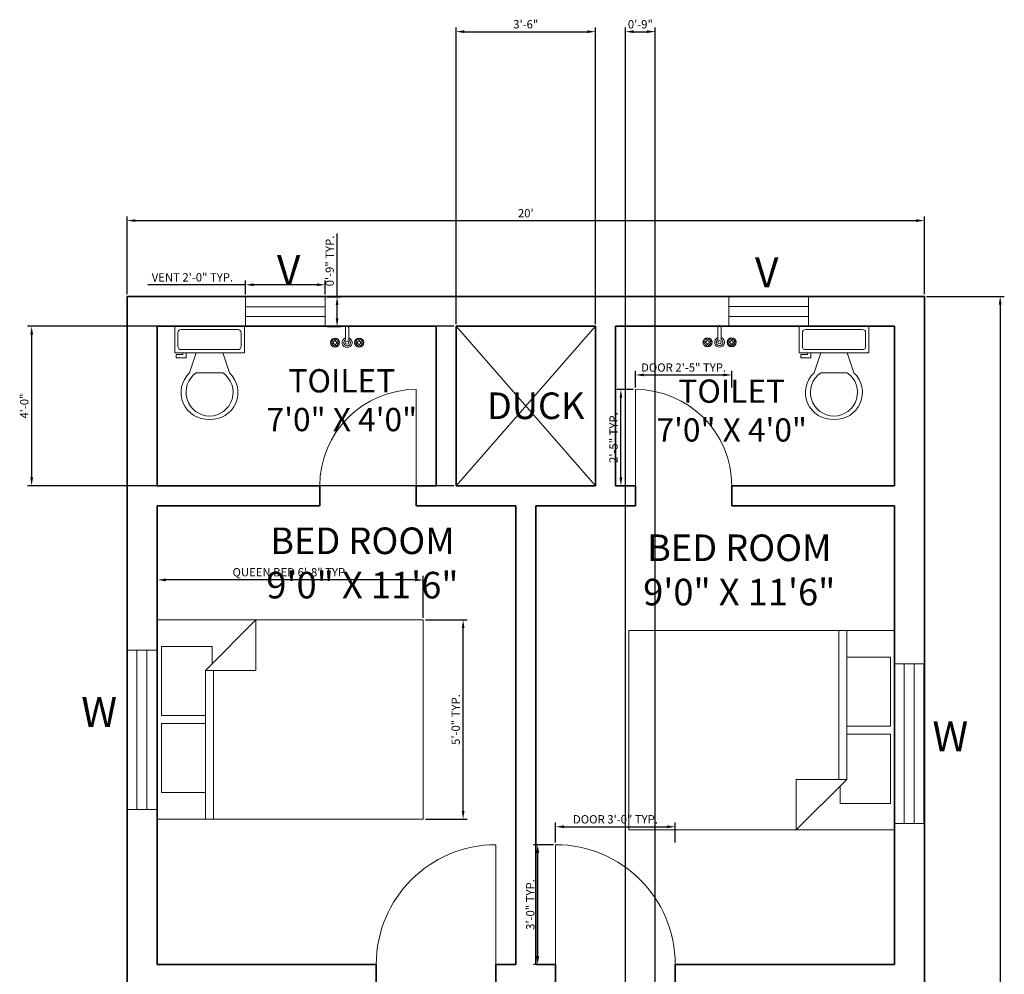
# Model space of a CAD drawing. Units: inches. Extents: x 1827 to 2455, y 1682 to 2281.
# Tile 3 of 3: x 2147 to 2443, y 1994 to 2281. Entities that reach past the tile are written whole.
import ezdxf

# ---------------------------------------------------------------- set-up
doc = ezdxf.new("R2010")
doc.units = ezdxf.units.IN
for name, color, linetype, lineweight in [('A-ANNO-DIMS', 2, 'Continuous', 18), ('A-ANNO-TEXT', 7, 'Continuous', 18), ('A-AREA-IDEN', 7, 'Continuous', 18), ('A-DOOR', 3, 'Continuous', 18), ('A-FLOR-FIXT', 9, 'Continuous', 18), ('A-FLOR-OPEN', 8, 'Continuous', 13), ('A-FURN', 8, 'Continuous', 18), ('A-GLAZ', 4, 'Continuous', 18), ('A-WALL', 7, 'Continuous', 35)]:
    doc.layers.add(name, color=color, linetype=linetype, lineweight=lineweight)
doc.styles.get("Standard").update_dxf_attribs({"font": 'arial.ttf'})
doc.dimstyles.new('ISO-25', dxfattribs={"dimtxt": 2.5, "dimasz": 2.5, "dimexe": 1.25, "dimexo": 0.625, "dimtad": 1, "dimdec": 0, "dimlunit": 3, "dimtxsty": 'Standard', "dimcen": 2.5, "dimadec": 0, "dimazin": 0, "dimtfac": 1, "dimtdec": 0, "dimtmove": 0, "dimatfit": 3, "dimfxl": 1, "dimarcsym": 0})

# ---------------------------------------------------------------- blocks, each defined once
blk = doc.blocks.new('Faucet - Bathroom top')
for p, q in [((-4.107, 0.125), (-4.375, 0.125)), ((-3.75, 0.4788), (-3.75, 0.75)), ((-3.5, 0.482), (-3.5, 0.75)), ((-3.1461, 0.125), (-2.875, 0.125)), ((3.143, 0.125), (2.875, 0.125)), ((3.5, 0.4788), (3.5, 0.75)), ((3.75, 0.482), (3.75, 0.75)), ((4.1039, 0.125), (4.375, 0.125)), ((-4.1039, -0.125), (-4.375, -0.125)), ((-3.75, -0.4821), (-3.75, -0.75)), ((-3.5, -0.4789), (-3.5, -0.75)), ((-3.143, -0.125), (-2.875, -0.125)), ((-0.5, -0.8639), (-0.5, -4.5)), ((0.5, -4.5), (0.5, -0.8631)), ((3.1461, -0.125), (2.875, -0.125)), ((3.5, -0.4821), (3.5, -0.75)), ((3.75, -0.4789), (3.75, -0.75)), ((4.107, -0.125), (4.375, -0.125))]:
    blk.add_line(p, q)
for centre, radius in [((-3.625, 0), 1.375), ((-4.625, 0), 0.2795), ((-3.625, 0), 0.5), ((-3.625, 1), 0.2795), ((-2.625, 0), 0.2795), ((0, 0), 0.5), ((3.625, 0), 1.375), ((2.625, 0), 0.2795), ((3.625, 0), 0.5), ((3.625, 1), 0.2795), ((4.625, 0), 0.2795), ((-3.625, -1), 0.2795), ((3.625, -1), 0.2795)]:
    blk.add_circle(centre, radius)
for centre, radius, start, end in [((-3.625, 0), 1, 105.2407, 164.2093), ((-3.625, 0), 1, 16.44125, 74.07887), ((0, 0), 1.5, 289.6514, 250.3603), ((0, 0), 1, 300.3431, 239.7554), ((3.625, 0), 1, 106.12, 164.0884), ((3.625, 0), 1, 16.23422, 73.90469), ((-3.625, 0), 1, 196.2342, 253.9047), ((-3.625, 0), 1, 286.12, 344.0884), ((3.625, 0), 1, 196.4413, 254.0789), ((3.625, 0), 1, 285.2407, 344.2093), ((0, -4.5), 0.5, 180, 0)]:
    blk.add_arc(centre, radius, start, end)
blk = doc.blocks.new('*U14')
for p, q in [((9.5, -6), (9.5, -2)), ((-10, -8.5), (-8, -8.5)), ((-10, -9.5), (-10, -8.5)), ((-8, -8.5), (-8, -8)), ((-7, -8), (-7, -9.5)), ((-4, -8), (-6, -14)), ((4, -8), (6, -14)), ((-7, -9.5), (-10, -9.5)), ((4, -14), (-4, -14))]:
    blk.add_line(p, q)
blk.add_lwpolyline([(10.5, -8), (10.5, 0), (-10.5, 0), (-10.5, -8)], close=True)
for points in [[(-9.5, -2), (-9.5, -6)], [(8.5, -1), (-8.5, -1)], [(-8.5, -7), (8.5, -7)]]:
    blk.add_lwpolyline(points)
for centre, radius, start, end in [((-8.625, -1.875), 0.8839, 81.8699, 188.1301), ((8.625, -1.875), 0.8839, 351.8699, 98.1301), ((-8.625, -6.125), 0.8839, 171.869898, 278.1301), ((8.625, -6.125), 0.8839, 261.8699, 8.1301), ((-0.4772, -19.9188), 8.0953, 133.01722, 273.38), ((0.0374, -19.8731), 7.127, 124.50543, 269.7), ((-0.0373, -19.8731), 7.127, 270.3, 55.4946), ((0.4773, -19.9188), 8.0953, 266.62, 46.9828)]:
    blk.add_arc(centre, radius, start, end)
blk = doc.blocks.new('Bed - Queen')
for p, q in [((0, -80.00003), (0, 0)), ((0, 0), (59.99999, 0)), ((59.99999, 0), (59.99999, -80.00003)), ((7.99999, -1.2), (28.79998, -1.2)), ((7.99999, -14.4), (7.99999, -1.2)), ((28.79998, -1.2), (28.79998, -14.4)), ((31.19999, -1.2), (51.99999, -1.2)), ((31.19999, -14.4), (31.19999, -1.2)), ((51.99999, -1.2), (51.99999, -16.4)), ((0, -14.4), (44.8, -14.4)), ((59.99999, -29.6), (44.8, -14.4)), ((44.8, -14.4), (44.8, -29.6)), ((44.8, -16.8), (0, -16.8)), ((51.99999, -16.4), (46.79936, -16.4)), ((44.8, -29.6), (59.99999, -29.6)), ((59.99999, -80.00003), (0, -80.00003))]:
    blk.add_line(p, q)
blk = doc.blocks.new('*D15')
at = {"layer": 'A-ANNO-DIMS', "color": 0, "lineweight": -2, "transparency": 16777216}
for p, q in [((2179.36, 2198.55), (2179.36, 2221.97)), ((2181.86, 2220.72), (2416.86, 2220.72)), ((2419.36, 2198.55), (2419.36, 2221.97))]:
    blk.add_line(p, q, dxfattribs=at)
at = {"layer": 'A-ANNO-DIMS', "color": 0, "transparency": 16777216}
for points in [[(2181.86, 2221.14), (2181.86, 2220.31), (2179.36, 2220.72)], [(2416.86, 2221.14), (2416.86, 2220.31), (2419.36, 2220.72)]]:
    blk.add_solid(points, dxfattribs=at)
at = {"layer": 'Defpoints', "color": 0, "transparency": 16777216}
for p in [(2419.36, 2220.72), (2179.36, 2197.92), (2419.36, 2197.92)]:
    blk.add_point(p, dxfattribs=at)
at = {"layer": 'A-ANNO-DIMS', "color": 0, "transparency": 16777216, "insert": (2299.36, 2222.63), "char_height": 2.5, "attachment_point": 5}
blk.add_mtext("20'", dxfattribs=at)
blk = doc.blocks.new('*D16')
at = {"layer": 'A-ANNO-DIMS', "color": 0, "lineweight": -2, "transparency": 16777216}
for p, q in [((2419.98, 2197.92), (2443.42, 2197.92)), ((2442.17, 2195.42), (2442.17, 1720.42)), ((2419.98, 1717.92), (2443.42, 1717.92))]:
    blk.add_line(p, q, dxfattribs=at)
at = {"layer": 'A-ANNO-DIMS', "color": 0, "transparency": 16777216}
for points in [[(2441.75, 2195.42), (2442.59, 2195.42), (2442.17, 2197.92)], [(2441.75, 1720.42), (2442.59, 1720.42), (2442.17, 1717.92)]]:
    blk.add_solid(points, dxfattribs=at)
at = {"layer": 'Defpoints', "color": 0, "transparency": 16777216}
for p in [(2419.36, 2197.92), (2419.36, 1717.92), (2442.17, 1717.92)]:
    blk.add_point(p, dxfattribs=at)
at = {"layer": 'A-ANNO-DIMS', "color": 0, "transparency": 16777216, "insert": (2440.27, 1957.92), "char_height": 2.5, "attachment_point": 5, "rotation": 90}
blk.add_mtext("40'", dxfattribs=at)
blk = doc.blocks.new('WIN-48IN')
for p, q in [((48, 9), (0, 9)), ((0, 9), (0, 0)), ((48, 0), (48, 9)), ((48, 6), (0, 6)), ((0, 3), (48, 3)), ((0, 0), (48, 0))]:
    blk.add_line(p, q)
blk = doc.blocks.new('VENT-24IN')
for p, q in [((0, 24), (0, 0)), ((0, 24), (9, 24)), ((3, 24), (3, 0)), ((6, 0), (6, 24)), ((9, 0), (9, 24)), ((0, 0), (9, 0))]:
    blk.add_line(p, q)
blk = doc.blocks.new('DOOR-29IN-SINGLE')
blk.add_line((0, 0), (0, 29))
blk.add_arc((0, 0), 29, 0, 90)
blk = doc.blocks.new('DOOR-36IN-SINGLE')
blk.add_line((0, 0), (0, 36))
blk.add_arc((0, 0), 36, 0, 90)
blk = doc.blocks.new('*D29')
at = {"layer": 'A-ANNO-DIMS', "color": 0, "lineweight": -2, "transparency": 16777216}
for p, q in [((2214.97, 2198.45), (2214.97, 2202.67)), ((2238.97, 2198.45), (2238.97, 2202.67)), ((2214.97, 2201.42), (2185.56, 2201.42)), ((2236.47, 2201.42), (2217.47, 2201.42))]:
    blk.add_line(p, q, dxfattribs=at)
at = {"layer": 'A-ANNO-DIMS', "color": 0, "transparency": 16777216}
for points in [[(2217.47, 2201.84), (2217.47, 2201.01), (2214.97, 2201.42)], [(2236.47, 2201.84), (2236.47, 2201.01), (2238.97, 2201.42)]]:
    blk.add_solid(points, dxfattribs=at)
at = {"layer": 'Defpoints', "color": 0, "transparency": 16777216}
for p in [(2214.97, 2201.42), (2214.97, 2197.82), (2238.97, 2197.82)]:
    blk.add_point(p, dxfattribs=at)
at = {"layer": 'A-ANNO-DIMS', "color": 0, "transparency": 16777216, "insert": (2199.01, 2203.32), "char_height": 2.5, "attachment_point": 5}
blk.add_mtext('VENT 2\'-0" TYP.', dxfattribs=at)
blk = doc.blocks.new('*D30')
at = {"layer": 'A-ANNO-DIMS', "color": 0, "lineweight": -2, "transparency": 16777216}
for p, q in [((2242.57, 2197.82), (2242.57, 2216.81)), ((2239.59, 2197.82), (2243.82, 2197.82)), ((2242.57, 2191.32), (2242.57, 2195.32)), ((2239.59, 2188.82), (2243.82, 2188.82))]:
    blk.add_line(p, q, dxfattribs=at)
at = {"layer": 'A-ANNO-DIMS', "color": 0, "transparency": 16777216}
for points in [[(2242.15, 2195.32), (2242.98, 2195.32), (2242.57, 2197.82)], [(2242.15, 2191.32), (2242.98, 2191.32), (2242.57, 2188.82)]]:
    blk.add_solid(points, dxfattribs=at)
at = {"layer": 'Defpoints', "color": 0, "transparency": 16777216}
for p in [(2238.97, 2197.82), (2242.57, 2197.82), (2238.97, 2188.82)]:
    blk.add_point(p, dxfattribs=at)
at = {"layer": 'A-ANNO-DIMS', "color": 0, "transparency": 16777216, "insert": (2240.66, 2208.57), "char_height": 2.5, "attachment_point": 5, "rotation": 90}
blk.add_mtext('0\'-9" TYP.', dxfattribs=at)
blk = doc.blocks.new('*D31')
at = {"layer": 'A-ANNO-DIMS', "color": 0, "lineweight": -2, "transparency": 16777216}
for p, q in [((2188.51, 2101.22), (2188.51, 2113.84)), ((2268.51, 2101.22), (2268.51, 2113.84)), ((2266.01, 2112.59), (2191.01, 2112.59))]:
    blk.add_line(p, q, dxfattribs=at)
at = {"layer": 'A-ANNO-DIMS', "color": 0, "transparency": 16777216}
for points in [[(2191.01, 2113.01), (2191.01, 2112.18), (2188.51, 2112.59)], [(2266.01, 2113.01), (2266.01, 2112.18), (2268.51, 2112.59)]]:
    blk.add_solid(points, dxfattribs=at)
at = {"layer": 'Defpoints', "color": 0, "transparency": 16777216}
for p in [(2188.51, 2112.59), (2188.51, 2100.59), (2268.51, 2100.59)]:
    blk.add_point(p, dxfattribs=at)
at = {"layer": 'A-ANNO-DIMS', "color": 0, "transparency": 16777216, "insert": (2228.51, 2114.59), "char_height": 2.5, "attachment_point": 5}
blk.add_mtext('QUEEN BED 6\'-8" TYP.', dxfattribs=at)
blk = doc.blocks.new('*D32')
at = {"layer": 'A-ANNO-DIMS', "color": 0, "lineweight": -2, "transparency": 16777216}
for p, q in [((2269.13, 2100.59), (2281.76, 2100.59)), ((2280.51, 2043.09), (2280.51, 2098.09)), ((2269.13, 2040.59), (2281.76, 2040.59))]:
    blk.add_line(p, q, dxfattribs=at)
at = {"layer": 'A-ANNO-DIMS', "color": 0, "transparency": 16777216}
for points in [[(2280.09, 2098.09), (2280.93, 2098.09), (2280.51, 2100.59)], [(2280.09, 2043.09), (2280.93, 2043.09), (2280.51, 2040.59)]]:
    blk.add_solid(points, dxfattribs=at)
at = {"layer": 'Defpoints', "color": 0, "transparency": 16777216}
for p in [(2268.51, 2100.59), (2280.51, 2100.59), (2268.51, 2040.59)]:
    blk.add_point(p, dxfattribs=at)
at = {"layer": 'A-ANNO-DIMS', "color": 0, "transparency": 16777216, "insert": (2278.61, 2070.59), "char_height": 2.5, "attachment_point": 5, "rotation": 90}
blk.add_mtext('5\'-0" TYP.', dxfattribs=at)
blk = doc.blocks.new('*D41')
at = {"layer": 'A-ANNO-DIMS', "color": 0, "lineweight": -2, "transparency": 16777216}
for p, q in [((2332.36, 2170.55), (2332.36, 2175.52)), ((2334.86, 2174.27), (2358.86, 2174.27)), ((2361.36, 2170.55), (2361.36, 2175.52))]:
    blk.add_line(p, q, dxfattribs=at)
at = {"layer": 'A-ANNO-DIMS', "color": 0, "transparency": 16777216}
for points in [[(2334.86, 2174.69), (2334.86, 2173.86), (2332.36, 2174.27)], [(2358.86, 2174.69), (2358.86, 2173.86), (2361.36, 2174.27)]]:
    blk.add_solid(points, dxfattribs=at)
at = {"layer": 'Defpoints', "color": 0, "transparency": 16777216}
for p in [(2361.36, 2174.27), (2332.36, 2169.92), (2361.36, 2169.92)]:
    blk.add_point(p, dxfattribs=at)
at = {"layer": 'A-ANNO-DIMS', "color": 0, "transparency": 16777216, "insert": (2346.86, 2176.19), "char_height": 2.5, "attachment_point": 5}
blk.add_mtext('DOOR 2\'-5" TYP.', dxfattribs=at)
blk = doc.blocks.new('*D42')
at = {"layer": 'A-ANNO-DIMS', "color": 0, "lineweight": -2, "transparency": 16777216}
for p, q in [((2331.73, 2169.92), (2326.76, 2169.92)), ((2328.01, 2143.42), (2328.01, 2167.42)), ((2331.73, 2140.92), (2326.76, 2140.92))]:
    blk.add_line(p, q, dxfattribs=at)
at = {"layer": 'A-ANNO-DIMS', "color": 0, "transparency": 16777216}
for points in [[(2327.59, 2167.42), (2328.42, 2167.42), (2328.01, 2169.92)], [(2327.59, 2143.42), (2328.42, 2143.42), (2328.01, 2140.92)]]:
    blk.add_solid(points, dxfattribs=at)
at = {"layer": 'Defpoints', "color": 0, "transparency": 16777216}
for p in [(2328.01, 2169.92), (2332.36, 2169.92), (2332.36, 2140.92)]:
    blk.add_point(p, dxfattribs=at)
at = {"layer": 'A-ANNO-DIMS', "color": 0, "transparency": 16777216, "insert": (2326.1, 2155.42), "char_height": 2.5, "attachment_point": 5, "rotation": 90}
blk.add_mtext('2\'-5" TYP.', dxfattribs=at)
blk = doc.blocks.new('*D43')
at = {"layer": 'A-ANNO-DIMS', "color": 0, "lineweight": -2, "transparency": 16777216}
for p, q in [((2308.36, 2033.55), (2308.36, 2039.57)), ((2344.36, 2033.55), (2344.36, 2039.57)), ((2310.86, 2038.32), (2341.86, 2038.32))]:
    blk.add_line(p, q, dxfattribs=at)
at = {"layer": 'A-ANNO-DIMS', "color": 0, "transparency": 16777216}
for points in [[(2310.86, 2038.74), (2310.86, 2037.91), (2308.36, 2038.32)], [(2341.86, 2038.74), (2341.86, 2037.91), (2344.36, 2038.32)]]:
    blk.add_solid(points, dxfattribs=at)
at = {"layer": 'Defpoints', "color": 0, "transparency": 16777216}
for p in [(2344.36, 2038.32), (2308.36, 2032.92), (2344.36, 2032.92)]:
    blk.add_point(p, dxfattribs=at)
at = {"layer": 'A-ANNO-DIMS', "color": 0, "transparency": 16777216, "insert": (2326.36, 2040.24), "char_height": 2.5, "attachment_point": 5}
blk.add_mtext('DOOR 3\'-0" TYP.', dxfattribs=at)
blk = doc.blocks.new('*D44')
at = {"layer": 'A-ANNO-DIMS', "color": 0, "lineweight": -2, "transparency": 16777216}
for p, q in [((2307.73, 2032.92), (2301.71, 2032.92)), ((2302.96, 1999.42), (2302.96, 2030.42)), ((2307.73, 1996.92), (2301.71, 1996.92))]:
    blk.add_line(p, q, dxfattribs=at)
at = {"layer": 'A-ANNO-DIMS', "color": 0, "transparency": 16777216}
for points in [[(2302.54, 2030.42), (2303.37, 2030.42), (2302.96, 2032.92)], [(2302.54, 1999.42), (2303.37, 1999.42), (2302.96, 1996.92)]]:
    blk.add_solid(points, dxfattribs=at)
at = {"layer": 'Defpoints', "color": 0, "transparency": 16777216}
for p in [(2302.96, 2032.92), (2308.36, 2032.92), (2308.36, 1996.92)]:
    blk.add_point(p, dxfattribs=at)
at = {"layer": 'A-ANNO-DIMS', "color": 0, "transparency": 16777216, "insert": (2301.05, 2014.92), "char_height": 2.5, "attachment_point": 5, "rotation": 90}
blk.add_mtext('3\'-0" TYP.', dxfattribs=at)
blk = doc.blocks.new('*D53')
at = {"layer": 'A-ANNO-DIMS', "color": 0, "lineweight": -2, "transparency": 16777216}
for p, q in [((2278.36, 2189.55), (2278.36, 2278.82)), ((2280.86, 2277.57), (2317.86, 2277.57)), ((2320.36, 2189.55), (2320.36, 2278.82))]:
    blk.add_line(p, q, dxfattribs=at)
at = {"layer": 'A-ANNO-DIMS', "color": 0, "transparency": 16777216}
for points in [[(2280.86, 2277.99), (2280.86, 2277.16), (2278.36, 2277.57)], [(2317.86, 2277.99), (2317.86, 2277.16), (2320.36, 2277.57)]]:
    blk.add_solid(points, dxfattribs=at)
at = {"layer": 'Defpoints', "color": 0, "transparency": 16777216}
for p in [(2320.36, 2277.57), (2278.36, 2188.92), (2320.36, 2188.92)]:
    blk.add_point(p, dxfattribs=at)
at = {"layer": 'A-ANNO-DIMS', "color": 0, "transparency": 16777216, "insert": (2299.36, 2279.47), "char_height": 2.5, "attachment_point": 5}
blk.add_mtext('3\'-6"', dxfattribs=at)
blk = doc.blocks.new('*D54')
at = {"layer": 'A-ANNO-DIMS', "color": 0, "lineweight": -2, "transparency": 16777216}
for p, q in [((2277.73, 2188.92), (2149.37, 2188.92)), ((2150.62, 2186.42), (2150.62, 2143.42)), ((2277.73, 2140.92), (2149.37, 2140.92))]:
    blk.add_line(p, q, dxfattribs=at)
at = {"layer": 'A-ANNO-DIMS', "color": 0, "transparency": 16777216}
for points in [[(2150.2, 2186.42), (2151.04, 2186.42), (2150.62, 2188.92)], [(2150.2, 2143.42), (2151.04, 2143.42), (2150.62, 2140.92)]]:
    blk.add_solid(points, dxfattribs=at)
at = {"layer": 'Defpoints', "color": 0, "transparency": 16777216}
for p in [(2278.36, 2188.92), (2150.62, 2140.92), (2278.36, 2140.92)]:
    blk.add_point(p, dxfattribs=at)
at = {"layer": 'A-ANNO-DIMS', "color": 0, "transparency": 16777216, "insert": (2148.72, 2164.92), "char_height": 2.5, "attachment_point": 5, "rotation": 90}
blk.add_mtext('4\'-0"', dxfattribs=at)
blk = doc.blocks.new('*D56')
at = {"layer": 'A-ANNO-DIMS', "color": 0, "lineweight": -2, "transparency": 16777216}
for p, q in [((2329.36, 1919.55), (2329.36, 2278.82)), ((2331.86, 2277.57), (2335.86, 2277.57)), ((2338.36, 1919.55), (2338.36, 2278.82))]:
    blk.add_line(p, q, dxfattribs=at)
at = {"layer": 'A-ANNO-DIMS', "color": 0, "transparency": 16777216}
for points in [[(2331.86, 2277.99), (2331.86, 2277.16), (2329.36, 2277.57)], [(2335.86, 2277.99), (2335.86, 2277.16), (2338.36, 2277.57)]]:
    blk.add_solid(points, dxfattribs=at)
at = {"layer": 'Defpoints', "color": 0, "transparency": 16777216}
for p in [(2338.36, 2277.57), (2329.36, 1918.92), (2338.36, 1918.92)]:
    blk.add_point(p, dxfattribs=at)
at = {"layer": 'A-ANNO-DIMS', "color": 0, "transparency": 16777216, "insert": (2333.86, 2279.47), "char_height": 2.5, "attachment_point": 5}
blk.add_mtext('0\'-9"', dxfattribs=at)

msp = doc.modelspace()

# ---------------------------------------------------------------- linework, layer by layer
at = {"layer": 'A-FLOR-OPEN'}
for p, q in [((2278.36, 2188.92), (2320.36, 2140.92)), ((2320.36, 2188.92), (2278.36, 2140.92)), ((2320.36, 2140.92), (2320.36, 2188.92))]:
    msp.add_line(p, q, dxfattribs=at)
at = {"layer": 'A-WALL'}
for p, q in [((2179.36, 2197.92), (2179.36, 1717.92)), ((2419.36, 2197.92), (2179.36, 2197.92)), ((2419.36, 1717.92), (2419.36, 2197.92)), ((2188.36, 2188.92), (2188.36, 2140.92)), ((2272.36, 2188.92), (2188.36, 2188.92)), ((2272.36, 2188.92), (2272.36, 2140.92)), ((2278.36, 2188.92), (2278.36, 2140.92)), ((2320.36, 2188.92), (2278.36, 2188.92)), ((2320.36, 2140.92), (2320.36, 2188.92)), ((2410.36, 2188.92), (2326.36, 2188.92)), ((2326.36, 2140.92), (2326.36, 2188.92)), ((2410.36, 2140.92), (2410.36, 2188.92)), ((2237.36, 2140.92), (2188.36, 2140.92)), ((2237.36, 2134.92), (2237.36, 2140.92)), ((2272.36, 2140.92), (2266.36, 2140.92)), ((2272.36, 2140.92), (2266.36, 2140.92)), ((2266.36, 2140.92), (2266.36, 2134.92)), ((2320.36, 2140.92), (2278.36, 2140.92)), ((2326.36, 2140.92), (2332.36, 2140.92)), ((2332.36, 2140.92), (2326.36, 2140.92)), ((2332.36, 2140.92), (2332.36, 2134.92)), ((2410.36, 2140.92), (2361.36, 2140.92)), ((2361.36, 2134.92), (2361.36, 2140.92)), ((2188.36, 2134.92), (2188.36, 1996.92)), ((2237.36, 2134.92), (2188.36, 2134.92)), ((2296.36, 2134.92), (2266.36, 2134.92)), ((2296.36, 1996.92), (2296.36, 2134.92)), ((2302.36, 2134.92), (2302.36, 1996.92)), ((2332.36, 2134.92), (2302.36, 2134.92)), ((2410.36, 2134.92), (2361.36, 2134.92)), ((2410.36, 1996.92), (2410.36, 2134.92)), ((2254.36, 1996.92), (2188.36, 1996.92)), ((2254.36, 1990.92), (2254.36, 1996.92)), ((2296.36, 1996.92), (2290.36, 1996.92)), ((2296.36, 1996.92), (2290.36, 1996.92)), ((2290.36, 1996.92), (2290.36, 1990.92)), ((2302.36, 1996.92), (2308.36, 1996.92)), ((2308.36, 1996.92), (2302.36, 1996.92)), ((2308.36, 1996.92), (2308.36, 1990.92)), ((2410.36, 1996.92), (2344.36, 1996.92)), ((2344.36, 1990.92), (2344.36, 1996.92))]:
    msp.add_line(p, q, dxfattribs=at)

# ---------------------------------------------------------------- block references
at = {"layer": 'A-DOOR', "extrusion": (0, 0, -1), "zscale": -1}
for name, p in [('DOOR-29IN-SINGLE', (-2266.36, 2140.92)), ('DOOR-36IN-SINGLE', (-2290.36, 1996.92))]:
    msp.add_blockref(name, p, dxfattribs=at)
at = {"layer": 'A-DOOR'}
for name, p in [('DOOR-29IN-SINGLE', (2332.36, 2140.92)), ('DOOR-36IN-SINGLE', (2308.36, 1996.92))]:
    msp.add_blockref(name, p, dxfattribs=at)
at = {"layer": 'A-FLOR-FIXT'}
for p in [(2204.17, 2188.92), (2392.14, 2188.92)]:
    msp.add_blockref('*U14', p, dxfattribs=at)
at = {"layer": 'A-FLOR-FIXT', "rotation": 180}
for p in [(2245.58, 2184.01), (2357.71, 2184.11)]:
    msp.add_blockref('Faucet - Bathroom top', p, dxfattribs=at)
at = {"layer": 'A-FURN'}
for p, rotation in [((2188.51, 2040.59), 89.99999999999999), ((2410.39, 2097.35), 270)]:
    msp.add_blockref('Bed - Queen', p, dxfattribs=dict(at, rotation=rotation))
at = {"layer": 'A-GLAZ'}
for name, p, rotation in [('VENT-24IN', (2238.97, 2188.82), 90.00000000000072), ('VENT-24IN', (2384.46, 2188.84), 89.99999999999477), ('WIN-48IN', (2188.27, 2043.49), 89.99999999999982), ('WIN-48IN', (2419.24, 2039.31), 89.99999999999895)]:
    msp.add_blockref(name, p, dxfattribs=dict(at, rotation=rotation))

# ---------------------------------------------------------------- texts
at = {"layer": 'A-ANNO-TEXT', "char_height": 9, "attachment_point": 1}
for s, width, insert in [('\\pxqc;V', 51.3012, (2202.33, 2210.36)), ('\\pxqc;V', 51.3012, (2346.25, 2209.62)), ('\\pxqc;W', 56.1832, (2142.85, 2077.34)), ('\\pxqc;W', 56.1832, (2399.07, 2070.06))]:
    msp.add_mtext_dynamic_manual_height_columns(s, width=width, gutter_width=12.5, heights=[0], dxfattribs=dict(at, insert=insert))
at = {"layer": 'A-AREA-IDEN', "attachment_point": 1}
for s, width, insert, char_height in [('\\pxqc;TOILET \\P7\'0" X 4\'0"', 49.9016, (2219.05, 2176.02), 7), ('\\pxqc;TOILET \\P7\'0" X 4\'0"', 49.9016, (2336.41, 2172.9), 7), ('\\pxqc;DUCK', 29.6325, (2287.54, 2169), 8), ('\\pxqc;BED ROOM \\P9\'0" X 11\'6"', 80.4211, (2209.98, 2128.37), 8), ('\\pxqc;BED ROOM ^J9\'0" X 11\'6"', 81.3384, (2322.96, 2126.27), 8)]:
    msp.add_mtext_dynamic_manual_height_columns(s, width=width, gutter_width=12.5, heights=[0], dxfattribs=dict(at, insert=insert, char_height=char_height))

# ---------------------------------------------------------------- dimensions: what is measured, and where the dimension line sits
at = {"layer": 'A-ANNO-DIMS'}
for base, p1, p2, override, picture, middle in [((2320.36, 2277.57), (2278.36, 2188.92), (2320.36, 2188.92), {"dimdec": 1, "dimlfac": 1, "dimrnd": 0, "dimzin": 1, "dimdsep": 46, "dimlunit": 4, "dimfrac": 2}, '*D53', (2299.36, 2279.47)), ((2338.36, 2277.57), (2329.36, 1918.92), (2338.36, 1918.92), {"dimdec": 1, "dimlfac": 1, "dimrnd": 0, "dimzin": 1, "dimdsep": 46, "dimlunit": 4, "dimfrac": 2}, '*D56', (2333.86, 2279.47)), ((2419.36, 2220.72), (2179.36, 2197.92), (2419.36, 2197.92), {"dimclrd": 0, "dimclre": 0, "dimclrt": 0}, '*D15', (2299.36, 2222.63))]:
    dim = msp.add_linear_dim(base=base, p1=p1, p2=p2, dimstyle='ISO-25', override=override, dxfattribs=at)
    dim.commit()
    dim.dimension.update_dxf_attribs({"geometry": picture, "text_midpoint": middle})
for base, p1, p2, angle, text, picture, middle in [((2242.57, 2197.82), (2238.97, 2188.82), (2238.97, 2197.82), 90, '<> TYP.', '*D30', (2240.66, 2208.57)), ((2214.97, 2201.42), (2238.97, 2197.82), (2214.97, 2197.82), 180, 'VENT <> TYP.', '*D29', (2199.01, 2203.32)), ((2328.01, 2169.92), (2332.36, 2140.92), (2332.36, 2169.92), 90, '<> TYP.', '*D42', (2326.1, 2155.42)), ((2188.51, 2112.59), (2268.51, 2100.59), (2188.51, 2100.59), 180, 'QUEEN BED <> TYP.', '*D31', (2228.51, 2114.59)), ((2280.51, 2100.59), (2268.51, 2040.59), (2268.51, 2100.59), 90, '<> TYP.', '*D32', (2278.61, 2070.59)), ((2302.96, 2032.92), (2308.36, 1996.92), (2308.36, 2032.92), 90, '<> TYP.', '*D44', (2301.05, 2014.92))]:
    dim = msp.add_linear_dim(base=base, p1=p1, p2=p2, angle=angle, text=text, dimstyle='ISO-25', override={"dimdec": 1, "dimlfac": 1, "dimrnd": 0, "dimzin": 1, "dimdsep": 46, "dimlunit": 4, "dimfrac": 2}, dxfattribs=at)
    dim.commit()
    dim.dimension.update_dxf_attribs({"geometry": picture, "text_midpoint": middle})
for base, p1, p2, override, picture, middle in [((2442.17, 1717.92), (2419.36, 2197.92), (2419.36, 1717.92), {"dimclrd": 0, "dimclre": 0, "dimclrt": 0}, '*D16', (2440.27, 1957.92)), ((2150.62, 2140.92), (2278.36, 2188.92), (2278.36, 2140.92), {"dimdec": 1, "dimlfac": 1, "dimrnd": 0, "dimzin": 1, "dimdsep": 46, "dimlunit": 4, "dimfrac": 2}, '*D54', (2148.72, 2164.92))]:
    dim = msp.add_linear_dim(base=base, p1=p1, p2=p2, angle=90, dimstyle='ISO-25', override=override, dxfattribs=at)
    dim.commit()
    dim.dimension.update_dxf_attribs({"geometry": picture, "text_midpoint": middle})
for base, p1, p2, picture, middle in [((2361.36, 2174.27), (2332.36, 2169.92), (2361.36, 2169.92), '*D41', (2346.86, 2176.19)), ((2344.36, 2038.32), (2308.36, 2032.92), (2344.36, 2032.92), '*D43', (2326.36, 2040.24))]:
    dim = msp.add_linear_dim(base=base, p1=p1, p2=p2, text='DOOR <> TYP.', dimstyle='ISO-25', override={"dimdec": 1, "dimlfac": 1, "dimrnd": 0, "dimzin": 1, "dimdsep": 46, "dimlunit": 4, "dimfrac": 2}, dxfattribs=at)
    dim.commit()
    dim.dimension.update_dxf_attribs({"geometry": picture, "text_midpoint": middle})

doc.saveas('drawing.dxf')
